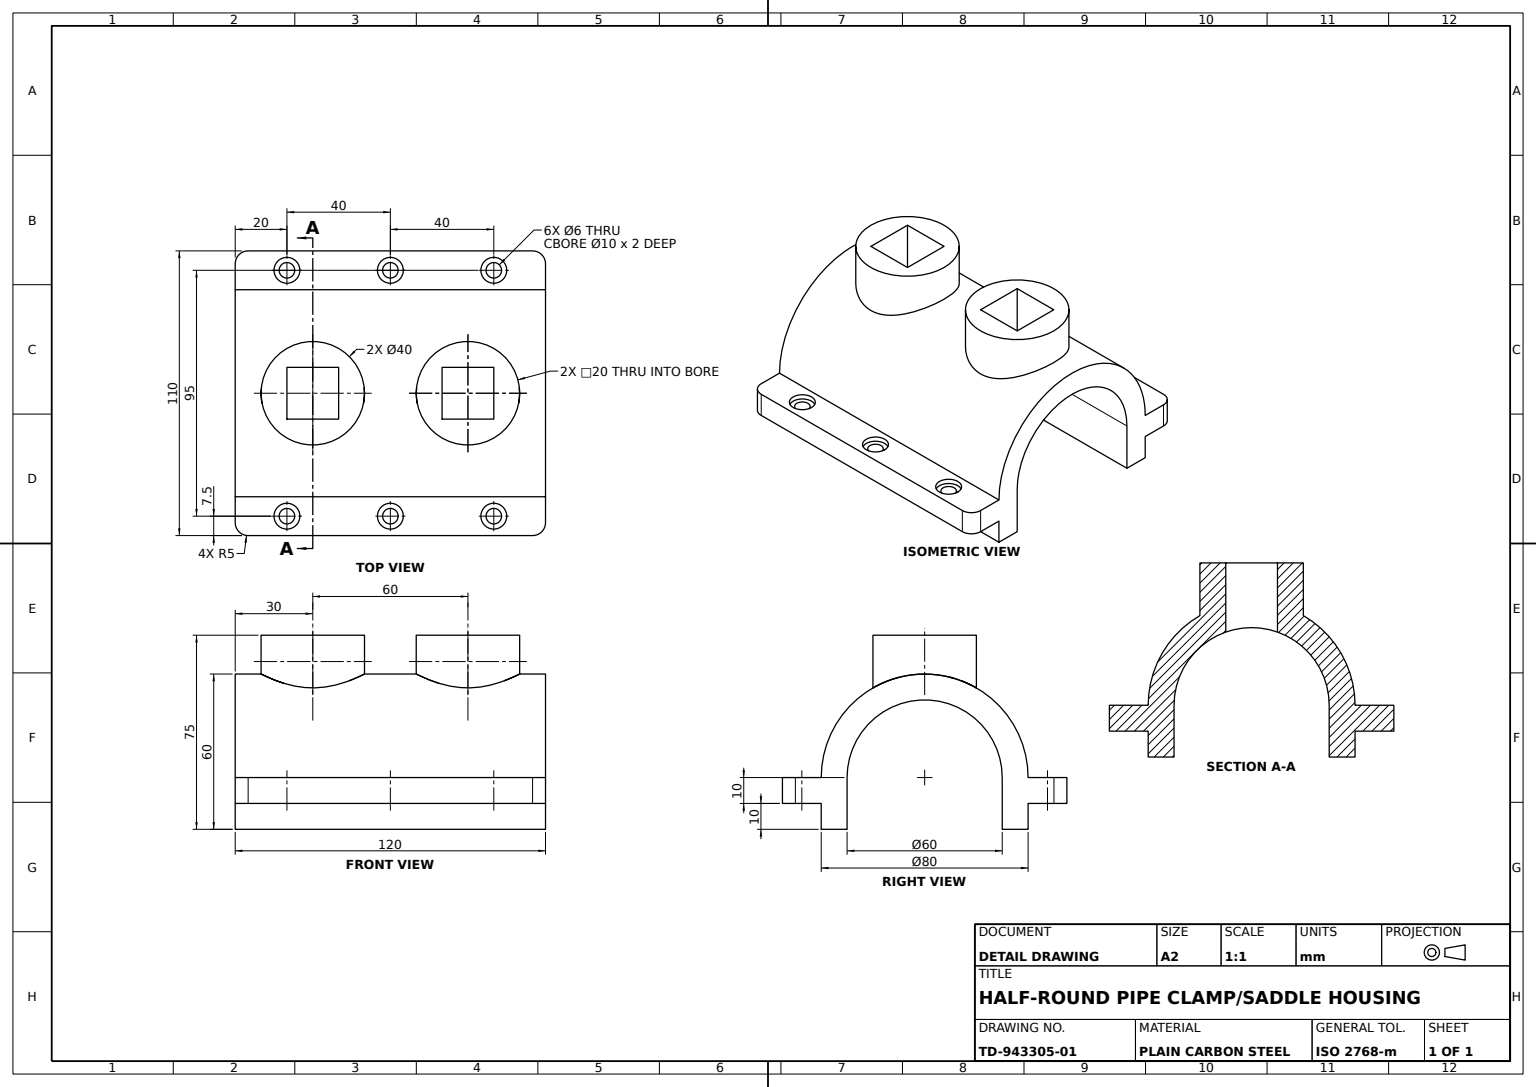
from build123d import *

# Parameters (mm, degrees)
SADDLE_BODY_DEPTH                       = 120
FLANGE_SKETCH_W                         = 15
FLANGE_SKETCH_H                         = 120
MOUNTING_FLANGE_DEPTH                   = 10
COUNTERBORED_FLANGE_HOLES_6_D           = 6
COUNTERBORED_FLANGE_HOLES_6_DEPTH       = 11.832159566
COUNTERBORED_FLANGE_HOLES_6_CBORE_D     = 10
COUNTERBORED_FLANGE_HOLES_6_CBORE_DEPTH = 2
TWIN_BOSSES_REACH                       = 153.822
TWIN_BOSSES_END_RADIUS                  = 40
TWIN_BOSS_SKETCH_R                      = 20
SQUARE_SOCKET_SKETCH_W                  = 20
SQUARE_SOCKET_SKETCH_H                  = 20
SQUARE_SOCKETS_20X20_DEPTH              = 152.822264586
FLANGE_FILLET_R5_R                      = 5


with BuildPart() as part:
    # Saddle Profile Sketch → Saddle Body (new body)
    with BuildSketch(Plane.XY):
        with BuildLine():
            Line((-40, 0), (-40, -20))
            Line((-40, -20), (-30, -20))
            Line((-30, -20), (-30, 0))
            ThreePointArc((-30, 0), (0, 30), (30, 0))
            Line((30, 0), (30, -20))
            Line((30, -20), (40, -20))
            Line((40, -20), (40, 0))
            ThreePointArc((40, 0), (0, 40), (-40, 0))
        make_face()
    extrude(amount=-SADDLE_BODY_DEPTH)

    # Flange Sketch → Mounting Flange (add)
    with BuildSketch(Plane(origin=(0, 0, 0), x_dir=(1, 0, 0), z_dir=(0, 1, 0))):
        with Locations((47.5, 60)):
            Rectangle(FLANGE_SKETCH_W, FLANGE_SKETCH_H)
        with Locations((-47.5, 60)):
            Rectangle(FLANGE_SKETCH_W, FLANGE_SKETCH_H)
    extrude(amount=-MOUNTING_FLANGE_DEPTH)

    # Counterbored Flange Holes Ø6
    with Locations(Plane(origin=(0, 0, 0), x_dir=(1, 0, 0), z_dir=(0, 1, 0))):
        with Locations((-47.5, 100), (-47.5, 60), (-47.5, 20), (47.5, 20), (47.5, 60), (47.5, 100)):
            CounterBoreHole(COUNTERBORED_FLANGE_HOLES_6_D / 2, COUNTERBORED_FLANGE_HOLES_6_CBORE_D / 2, COUNTERBORED_FLANGE_HOLES_6_CBORE_DEPTH, depth=COUNTERBORED_FLANGE_HOLES_6_DEPTH)

    # Twin Bosses: up to this cylinder (the profile starts outside it)
    twin_bosses_end = Plane(origin=(0, 0, -60), z_dir=(0, 0, 1)) * Cylinder(TWIN_BOSSES_END_RADIUS, 448.644, mode=Mode.PRIVATE)
    # Twin Boss Sketch → Twin Bosses (add, up to the surface)
    with BuildSketch(Plane(origin=(0, 55, 0), x_dir=(1, 0, 0), z_dir=(0, 1, 0)), mode=Mode.PRIVATE) as twin_bosses_sk1:
        with Locations(Location((0, 90, 0), (0, 0, 270))):
            Circle(TWIN_BOSS_SKETCH_R)
    twin_bosses_tool1 = extrude(twin_bosses_sk1.sketch, amount=-TWIN_BOSSES_REACH, mode=Mode.PRIVATE) - twin_bosses_end
    add(twin_bosses_tool1.solids().sort_by_distance((0, 55, -90))[0])
    # Twin Boss Sketch → Twin Bosses (add, up to the surface)
    with BuildSketch(Plane(origin=(0, 55, 0), x_dir=(1, 0, 0), z_dir=(0, 1, 0)), mode=Mode.PRIVATE) as twin_bosses_sk2:
        with Locations(Location((0, 30, 0), (0, 0, 270))):
            Circle(TWIN_BOSS_SKETCH_R)
    twin_bosses_tool2 = extrude(twin_bosses_sk2.sketch, amount=-TWIN_BOSSES_REACH, mode=Mode.PRIVATE) - twin_bosses_end
    add(twin_bosses_tool2.solids().sort_by_distance((0, 55, -30))[0])

    # Square Socket Sketch → Square Sockets 20x20 (cut, through all)
    with BuildSketch(Plane(origin=(0, 55, 0), x_dir=(1, 0, 0), z_dir=(0, 1, 0))):
        with Locations((0, 90)):
            Rectangle(SQUARE_SOCKET_SKETCH_W, SQUARE_SOCKET_SKETCH_H)
        with Locations((0, 30)):
            Rectangle(SQUARE_SOCKET_SKETCH_W, SQUARE_SOCKET_SKETCH_H)
    extrude(amount=-SQUARE_SOCKETS_20X20_DEPTH, mode=Mode.SUBTRACT)

    # Flange Fillet R5
    flange_fillet_r5_edges = [part.edges().sort_by_distance(p)[0] for p in [
        (55, -5, -120),
        (55, -5, 0),
        (-55, -5, 0),
        (-55, -5, -120),
    ]]
    fillet(flange_fillet_r5_edges, radius=FLANGE_FILLET_R5_R)


solid = part.part
